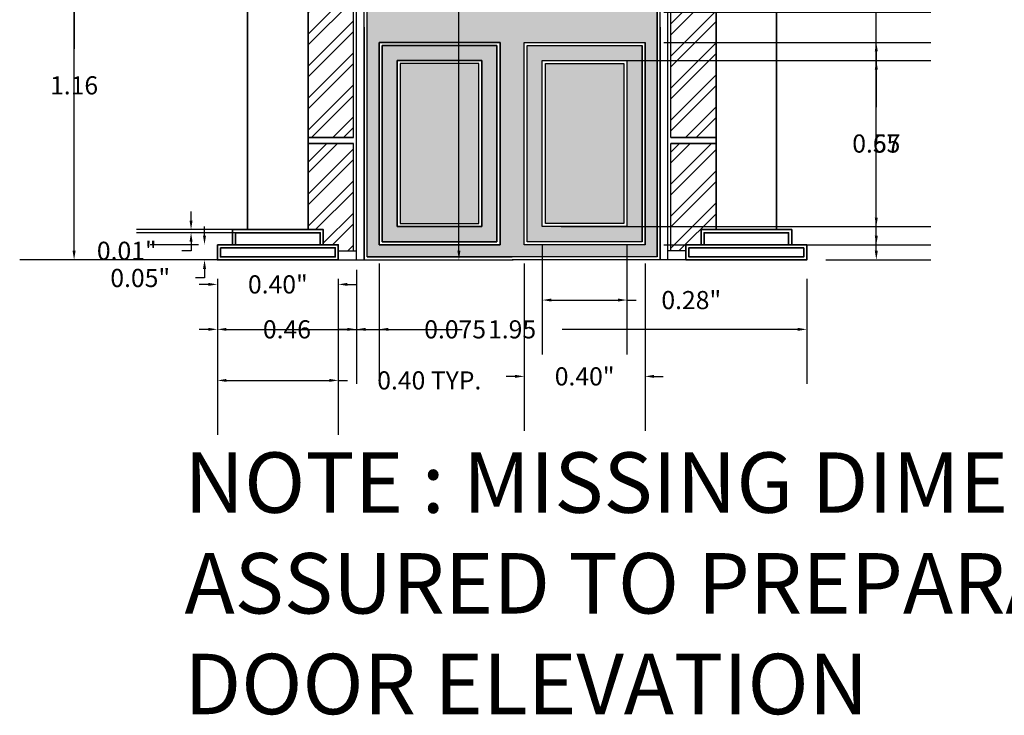
# Model space of a CAD drawing. Units: inches. Extents: x 19.36 to 24.97, y -1.46 to 4.09.
# Tile 1 of 4: x 19.36 to 22.62, y -1.46 to 0.85. Entities that reach past the tile are written whole.
import ezdxf

# ---------------------------------------------------------------- set-up
doc = ezdxf.new("R2010")
doc.units = ezdxf.units.IN
doc.header["$MEASUREMENT"] = 0
for name, color, linetype, lineweight in [('A-ANNO-DIMS', 2, 'Continuous', 18), ('A-ANNO-TEXT', 7, 'Continuous', 25), ('A-COLS', 3, 'Continuous', 35), ('A-DOOR', 4, 'Continuous', 25), ('A-ELEV', 7, 'Continuous', 35), ('A-ELEV-PATT', 8, 'Continuous', 13)]:
    doc.layers.add(name, color=color, linetype=linetype, lineweight=lineweight)
doc.styles.get("Standard").update_dxf_attribs({"font": 'arial.ttf'})
doc.dimstyles.get("Standard").update_dxf_attribs({"dimtxt": 0.06, "dimasz": 0.03, "dimexe": 0.18, "dimexo": 0.0625, "dimgap": 0.09, "dimtad": 0, "dimtih": 1, "dimtoh": 1, "dimzin": 0, "dimdsep": 46, "dimlunit": 3, "dimtxsty": 'Standard', "dimcen": 0, "dimadec": 0, "dimazin": 0, "dimtfac": 1, "dimtofl": 0, "dimtmove": 0, "dimatfit": 3, "dimfxl": 1, "dimtolj": 1, "dimtzin": 0, "dimarcsym": 1})

# ---------------------------------------------------------------- blocks, each defined once
blk = doc.blocks.new('*D10')
at = {"layer": 'A-ANNO-DIMS', "color": 0, "lineweight": -2, "transparency": 16777216}
for p, q in [((21.0886, 0.0975), (21.0886, -0.2631)), ((21.3686, 0.0975), (21.3686, -0.2631)), ((21.1186, -0.0831), (21.3386, -0.0831)), ((21.3686, -0.0831), (21.3986, -0.0831))]:
    blk.add_line(p, q, dxfattribs=at)
at = {"layer": 'A-ANNO-DIMS', "color": 0, "transparency": 16777216}
for points in [[(21.1186, -0.0781), (21.1186, -0.0881), (21.0886, -0.0831)], [(21.3386, -0.0781), (21.3386, -0.0881), (21.3686, -0.0831)]]:
    blk.add_solid(points, dxfattribs=at)
at = {"layer": 'Defpoints', "color": 0, "transparency": 16777216}
for p in [(21.0886, 0.16), (21.3686, 0.16), (21.3686, -0.0831)]:
    blk.add_point(p, dxfattribs=at)
at = {"layer": 'A-ANNO-DIMS', "color": 0, "transparency": 16777216, "insert": (21.5814, -0.0831), "char_height": 0.06, "width": 0.195629, "attachment_point": 5}
blk.add_mtext('\\A1;0.28"', dxfattribs=at)
blk = doc.blocks.new('*D11')
at = {"layer": 'A-ANNO-DIMS', "color": 0, "lineweight": -2, "transparency": 16777216}
for p, q in [((21.0286, 0.0375), (21.0286, -0.5157)), ((21.4286, 0.0375), (21.4286, -0.5157)), ((20.9986, -0.3357), (20.9686, -0.3357)), ((21.4586, -0.3357), (21.4886, -0.3357))]:
    blk.add_line(p, q, dxfattribs=at)
at = {"layer": 'A-ANNO-DIMS', "color": 0, "transparency": 16777216}
for points in [[(20.9986, -0.3307), (20.9986, -0.3407), (21.0286, -0.3357)], [(21.4586, -0.3307), (21.4586, -0.3407), (21.4286, -0.3357)]]:
    blk.add_solid(points, dxfattribs=at)
at = {"layer": 'Defpoints', "color": 0, "transparency": 16777216}
for p in [(21.0286, 0.1), (21.4286, 0.1), (21.4286, -0.3357)]:
    blk.add_point(p, dxfattribs=at)
at = {"layer": 'A-ANNO-DIMS', "color": 0, "transparency": 16777216, "insert": (21.2286, -0.3357), "char_height": 0.06, "attachment_point": 5}
blk.add_mtext('\\A1;0.40"', dxfattribs=at)
blk = doc.blocks.new('*D12')
at = {"layer": 'A-ANNO-DIMS', "color": 0, "lineweight": -2, "transparency": 16777216}
for p, q in [((19.9836, -0.0312), (19.9536, -0.0312)), ((20.0136, -0.0125), (20.0136, -0.2112)), ((20.4136, -0.0125), (20.4136, -0.2112)), ((20.4436, -0.0312), (20.4736, -0.0312))]:
    blk.add_line(p, q, dxfattribs=at)
at = {"layer": 'A-ANNO-DIMS', "color": 0, "transparency": 16777216}
for points in [[(19.9836, -0.0262), (19.9836, -0.0362), (20.0136, -0.0312)], [(20.4436, -0.0262), (20.4436, -0.0362), (20.4136, -0.0312)]]:
    blk.add_solid(points, dxfattribs=at)
at = {"layer": 'Defpoints', "color": 0, "transparency": 16777216}
for p in [(20.0136, 0.05), (20.4136, 0.05), (20.4136, -0.0312)]:
    blk.add_point(p, dxfattribs=at)
at = {"layer": 'A-ANNO-DIMS', "color": 0, "transparency": 16777216, "insert": (20.2136, -0.0312), "char_height": 0.06, "attachment_point": 5}
blk.add_mtext('\\A1;0.40"', dxfattribs=at)
blk = doc.blocks.new('*D13')
at = {"layer": 'A-ANNO-DIMS', "color": 0, "lineweight": -2, "transparency": 16777216}
for p, q in [((19.9709, 0.13), (19.9709, 0.16)), ((19.9511, 0.1), (19.7909, 0.1)), ((19.9511, 0.05), (19.7909, 0.05)), ((19.9709, 0.02), (19.9709, -0.01)), ((19.9709, -0.01), (19.9409, -0.01))]:
    blk.add_line(p, q, dxfattribs=at)
at = {"layer": 'A-ANNO-DIMS', "color": 0, "transparency": 16777216}
for points in [[(19.9659, 0.13), (19.9759, 0.13), (19.9709, 0.1)], [(19.9659, 0.02), (19.9759, 0.02), (19.9709, 0.05)]]:
    blk.add_solid(points, dxfattribs=at)
at = {"layer": 'Defpoints', "color": 0, "transparency": 16777216}
for p in [(20.0136, 0.1), (19.9709, 0.05), (20.0136, 0.05)]:
    blk.add_point(p, dxfattribs=at)
at = {"layer": 'A-ANNO-DIMS', "color": 0, "transparency": 16777216, "insert": (19.7582, -0.01), "char_height": 0.06, "attachment_point": 5}
blk.add_mtext('\\A1;0.05"', dxfattribs=at)
blk = doc.blocks.new('*D14')
at = {"layer": 'A-ANNO-DIMS', "color": 0, "lineweight": -2, "transparency": 16777216}
for p, q in [((19.9264, 0.18), (19.9264, 0.21)), ((20.1322, 0.15), (19.7464, 0.15)), ((20.1322, 0.14), (19.7464, 0.14)), ((19.9264, 0.11), (19.9264, 0.08)), ((19.9264, 0.08), (19.8964, 0.08))]:
    blk.add_line(p, q, dxfattribs=at)
at = {"layer": 'A-ANNO-DIMS', "color": 0, "transparency": 16777216}
for points in [[(19.9214, 0.18), (19.9314, 0.18), (19.9264, 0.15)], [(19.9214, 0.11), (19.9314, 0.11), (19.9264, 0.14)]]:
    blk.add_solid(points, dxfattribs=at)
at = {"layer": 'Defpoints', "color": 0, "transparency": 16777216}
for p in [(19.9264, 0.14), (20.1947, 0.15), (20.1947, 0.14)]:
    blk.add_point(p, dxfattribs=at)
at = {"layer": 'A-ANNO-DIMS', "color": 0, "transparency": 16777216, "insert": (19.7137, 0.08), "char_height": 0.06, "attachment_point": 5}
blk.add_mtext('\\A1;0.01"', dxfattribs=at)
blk = doc.blocks.new('PILASTER')
for p, q in [((20.1136, 2.65), (20.0636, 2.65)), ((20.1136, 2.65), (20.0636, 2.65)), ((20.0636, 2.65), (20.0636, 2.62)), ((20.1136, 2.65), (20.3136, 2.65)), ((20.1136, 2.65), (20.3136, 2.65)), ((20.3136, 2.65), (20.3636, 2.65)), ((20.3136, 2.65), (20.3636, 2.65)), ((20.3636, 2.62), (20.3636, 2.65)), ((20.1136, 2.62), (20.0636, 2.62)), ((20.1136, 2.62), (20.0636, 2.62)), ((20.1136, 2.05), (20.1136, 2.62)), ((20.1136, 2.62), (20.3136, 2.62)), ((20.1136, 2.62), (20.3136, 2.62)), ((20.3136, 2.05), (20.3136, 2.62)), ((20.3136, 2.62), (20.3636, 2.62)), ((20.3136, 2.62), (20.3636, 2.62)), ((20.1136, 1.95), (20.0636, 1.95)), ((20.0636, 1.95), (20.0636, 1.92)), ((20.1136, 1.95), (20.3136, 1.95)), ((20.3136, 1.95), (20.3636, 1.95)), ((20.3636, 1.92), (20.3636, 1.95)), ((20.1136, 1.92), (20.0636, 1.92)), ((20.1136, 0.15), (20.1136, 1.92)), ((20.1136, 1.92), (20.3136, 1.92)), ((20.3136, 0.15), (20.3136, 1.92)), ((20.3136, 1.92), (20.3636, 1.92)), ((20.3136, 0.15), (20.3136, 0.32)), ((20.0636, 0.15), (20.1136, 0.15)), ((20.3636, 0.15), (20.3136, 0.15)), ((20.0136, 0.1), (20.0636, 0.1)), ((20.0136, 0.1), (20.0636, 0.1)), ((20.4136, 0.1), (20.3636, 0.1))]:
    blk.add_line(p, q)
blk.add_lwpolyline([(20.3636, 0.1), (20.3636, 0.15), (20.0636, 0.15), (20.0636, 0.1)])
blk.add_lwpolyline([(20.0136, 0.1), (20.4136, 0.1), (20.4136, 0.05), (20.0136, 0.05)], close=True)
for centre, start, end in [((20.0886, 2.71), 180, 247.3801), ((20.3386, 2.71), 292.6199, 0), ((20.0886, 2.01), 180, 247.3801), ((20.3386, 2.01), 292.6199, 0)]:
    blk.add_arc(centre, 0.065, start, end)
blk = doc.blocks.new('*D17')
at = {"layer": 'A-ANNO-DIMS', "color": 0, "lineweight": -2, "transparency": 16777216}
for p, q in [((20.4761, 2.71), (20.9926, 2.71)), ((20.8126, 2.68), (20.8126, 1.501)), ((20.8126, 0.08), (20.8126, 1.259)), ((20.4761, 0.05), (20.9926, 0.05))]:
    blk.add_line(p, q, dxfattribs=at)
at = {"layer": 'A-ANNO-DIMS', "color": 0, "transparency": 16777216}
for points in [[(20.8076, 2.68), (20.8176, 2.68), (20.8126, 2.71)], [(20.8076, 0.08), (20.8176, 0.08), (20.8126, 0.05)]]:
    blk.add_solid(points, dxfattribs=at)
at = {"layer": 'Defpoints', "color": 0, "transparency": 16777216}
for p in [(20.4136, 2.71), (20.8126, 2.71), (20.4136, 0.05)]:
    blk.add_point(p, dxfattribs=at)
at = {"layer": 'A-ANNO-DIMS', "color": 0, "transparency": 16777216, "insert": (20.8126, 1.38), "char_height": 0.06, "attachment_point": 5}
blk.add_mtext('\\A1;PILASTER 2.66 TYP.', dxfattribs=at)
blk = doc.blocks.new('*D18')
at = {"layer": 'A-ANNO-DIMS', "color": 0, "lineweight": -2, "transparency": 16777216}
for p, q in [((20.0136, -0.0125), (20.0136, -0.529)), ((20.4136, -0.0125), (20.4136, -0.529)), ((20.0436, -0.349), (20.3836, -0.349)), ((20.4136, -0.349), (20.4436, -0.349))]:
    blk.add_line(p, q, dxfattribs=at)
at = {"layer": 'A-ANNO-DIMS', "color": 0, "transparency": 16777216}
for points in [[(20.0436, -0.344), (20.0436, -0.354), (20.0136, -0.349)], [(20.3836, -0.344), (20.3836, -0.354), (20.4136, -0.349)]]:
    blk.add_solid(points, dxfattribs=at)
at = {"layer": 'Defpoints', "color": 0, "transparency": 16777216}
for p in [(20.0136, 0.05), (20.4136, 0.05), (20.4136, -0.349)]:
    blk.add_point(p, dxfattribs=at)
at = {"layer": 'A-ANNO-DIMS', "color": 0, "transparency": 16777216, "insert": (20.7146, -0.349), "char_height": 0.06, "attachment_point": 5}
blk.add_mtext('\\A1;0.40 TYP.', dxfattribs=at)
blk = doc.blocks.new('*D19')
at = {"layer": 'A-ANNO-DIMS', "color": 0, "lineweight": -2, "transparency": 16777216}
for p, q in [((20.0136, -0.0125), (20.0136, -0.36)), ((21.9636, -0.0125), (21.9636, -0.36)), ((20.0436, -0.18), (20.8233, -0.18)), ((21.9336, -0.18), (21.154, -0.18))]:
    blk.add_line(p, q, dxfattribs=at)
at = {"layer": 'A-ANNO-DIMS', "color": 0, "transparency": 16777216}
for points in [[(20.0436, -0.175), (20.0436, -0.185), (20.0136, -0.18)], [(21.9336, -0.175), (21.9336, -0.185), (21.9636, -0.18)]]:
    blk.add_solid(points, dxfattribs=at)
at = {"layer": 'Defpoints', "color": 0, "transparency": 16777216}
for p in [(20.0136, 0.05), (21.9636, 0.05), (21.9636, -0.18)]:
    blk.add_point(p, dxfattribs=at)
at = {"layer": 'A-ANNO-DIMS', "color": 0, "transparency": 16777216, "insert": (20.9886, -0.18), "char_height": 0.06, "attachment_point": 5}
blk.add_mtext('\\A1;1.95', dxfattribs=at)
blk = doc.blocks.new('*D20')
at = {"layer": 'A-ANNO-DIMS', "color": 0, "lineweight": -2, "transparency": 16777216}
for p, q in [((21.0509, 3.5451), (22.3736, 3.5451)), ((22.1936, 3.5151), (22.1936, 1.9182)), ((22.1936, 0.08), (22.1936, 1.6769)), ((22.0261, 0.05), (22.3736, 0.05))]:
    blk.add_line(p, q, dxfattribs=at)
at = {"layer": 'A-ANNO-DIMS', "color": 0, "transparency": 16777216}
for points in [[(22.1886, 3.5151), (22.1986, 3.5151), (22.1936, 3.5451)], [(22.1886, 0.08), (22.1986, 0.08), (22.1936, 0.05)]]:
    blk.add_solid(points, dxfattribs=at)
at = {"layer": 'Defpoints', "color": 0, "transparency": 16777216}
for p in [(20.9884, 3.5451), (22.1936, 3.5451), (21.9636, 0.05)]:
    blk.add_point(p, dxfattribs=at)
at = {"layer": 'A-ANNO-DIMS', "color": 0, "transparency": 16777216, "insert": (22.1936, 1.7976), "char_height": 0.06, "attachment_point": 5}
blk.add_mtext('\\A1;3.495', dxfattribs=at)
blk = doc.blocks.new('*D21')
at = {"layer": 'A-ANNO-DIMS', "color": 0, "lineweight": -2, "transparency": 16777216}
for p, q in [((20.4736, 0.1125), (20.4736, 4.0914)), ((21.5036, 0.1125), (21.5036, 4.0914)), ((20.5036, 3.9114), (20.8235, 3.9114)), ((21.4736, 3.9114), (21.1537, 3.9114))]:
    blk.add_line(p, q, dxfattribs=at)
at = {"layer": 'A-ANNO-DIMS', "color": 0, "transparency": 16777216}
for points in [[(20.5036, 3.9164), (20.5036, 3.9064), (20.4736, 3.9114)], [(21.4736, 3.9164), (21.4736, 3.9064), (21.5036, 3.9114)]]:
    blk.add_solid(points, dxfattribs=at)
at = {"layer": 'Defpoints', "color": 0, "transparency": 16777216}
for p in [(21.5036, 3.9114), (20.4736, 0.05), (21.5036, 0.05)]:
    blk.add_point(p, dxfattribs=at)
at = {"layer": 'A-ANNO-DIMS', "color": 0, "transparency": 16777216, "insert": (20.9886, 3.9114), "char_height": 0.06, "attachment_point": 5}
blk.add_mtext('\\A1;1.03', dxfattribs=at)
blk = doc.blocks.new('*D22')
at = {"layer": 'A-ANNO-DIMS', "color": 0, "lineweight": -2, "transparency": 16777216}
for p, q in [((20.013629, -0.012487), (20.013629, -0.359987)), ((20.473629, -0.012487), (20.473629, -0.359987)), ((19.983629, -0.179987), (19.953629, -0.179987)), ((20.503629, -0.179987), (20.533629, -0.179987))]:
    blk.add_line(p, q, dxfattribs=at)
at = {"layer": 'A-ANNO-DIMS', "color": 0, "transparency": 16777216}
for points in [[(19.983629, -0.174987), (19.983629, -0.184987), (20.013629, -0.179987)], [(20.503629, -0.174987), (20.503629, -0.184987), (20.473629, -0.179987)]]:
    blk.add_solid(points, dxfattribs=at)
at = {"layer": 'Defpoints', "color": 0, "transparency": 16777216}
for p in [(20.013629, 0.050013), (20.473629, 0.050013), (20.473629, -0.179987)]:
    blk.add_point(p, dxfattribs=at)
at = {"layer": 'A-ANNO-DIMS', "color": 0, "transparency": 16777216, "insert": (20.243629, -0.179987), "char_height": 0.06, "attachment_point": 5}
blk.add_mtext('\\A1;0.46', dxfattribs=at)
blk = doc.blocks.new('*D23')
at = {"layer": 'A-ANNO-DIMS', "color": 0, "lineweight": -2, "transparency": 16777216}
for p, q in [((20.9261, 1.2054), (19.3594, 1.2054)), ((19.5394, 1.1754), (19.5394, 0.7483)), ((19.5394, 0.08), (19.5394, 0.5071)), ((20.4111, 0.05), (19.3594, 0.05))]:
    blk.add_line(p, q, dxfattribs=at)
at = {"layer": 'A-ANNO-DIMS', "color": 0, "transparency": 16777216}
for points in [[(19.5344, 1.1754), (19.5444, 1.1754), (19.5394, 1.2054)], [(19.5344, 0.08), (19.5444, 0.08), (19.5394, 0.05)]]:
    blk.add_solid(points, dxfattribs=at)
at = {"layer": 'Defpoints', "color": 0, "transparency": 16777216}
for p in [(19.5394, 1.2054), (20.9886, 1.2054), (20.4736, 0.05)]:
    blk.add_point(p, dxfattribs=at)
at = {"layer": 'A-ANNO-DIMS', "color": 0, "transparency": 16777216, "insert": (19.5394, 0.6277), "char_height": 0.06, "attachment_point": 5}
blk.add_mtext('\\A1;1.16', dxfattribs=at)
blk = doc.blocks.new('*D26')
at = {"layer": 'A-ANNO-DIMS', "color": 0, "lineweight": -2, "transparency": 16777216}
for p, q in [((19.9511, 2.75), (19.3594, 2.75)), ((19.5394, 2.72), (19.5394, 1.5206)), ((19.5394, 0.08), (19.5394, 1.2794)), ((19.9511, 0.05), (19.3594, 0.05))]:
    blk.add_line(p, q, dxfattribs=at)
at = {"layer": 'A-ANNO-DIMS', "color": 0, "transparency": 16777216}
for points in [[(19.5344, 2.72), (19.5444, 2.72), (19.5394, 2.75)], [(19.5344, 0.08), (19.5444, 0.08), (19.5394, 0.05)]]:
    blk.add_solid(points, dxfattribs=at)
at = {"layer": 'Defpoints', "color": 0, "transparency": 16777216}
for p in [(19.5394, 2.75), (20.0136, 2.75), (20.0136, 0.05)]:
    blk.add_point(p, dxfattribs=at)
at = {"layer": 'A-ANNO-DIMS', "color": 0, "transparency": 16777216, "insert": (19.5394, 1.4), "char_height": 0.06, "attachment_point": 5}
blk.add_mtext('\\A1;2.70', dxfattribs=at)
blk = doc.blocks.new('*D27')
at = {"layer": 'A-ANNO-DIMS', "color": 0, "lineweight": -2, "transparency": 16777216}
for p, q in [((19.9523, 2.9877), (19.3594, 2.9877)), ((19.5394, 2.9577), (19.5394, 1.6395)), ((19.5394, 0.08), (19.5394, 1.3982)), ((19.9511, 0.05), (19.3594, 0.05))]:
    blk.add_line(p, q, dxfattribs=at)
at = {"layer": 'A-ANNO-DIMS', "color": 0, "transparency": 16777216}
for points in [[(19.5344, 2.9577), (19.5444, 2.9577), (19.5394, 2.9877)], [(19.5344, 0.08), (19.5444, 0.08), (19.5394, 0.05)]]:
    blk.add_solid(points, dxfattribs=at)
at = {"layer": 'Defpoints', "color": 0, "transparency": 16777216}
for p in [(20.0148, 2.9877), (19.5394, 0.05), (20.0136, 0.05)]:
    blk.add_point(p, dxfattribs=at)
at = {"layer": 'A-ANNO-DIMS', "color": 0, "transparency": 16777216, "insert": (19.5394, 1.5189), "char_height": 0.06, "attachment_point": 5}
blk.add_mtext('\\A1;2.938', dxfattribs=at)
blk = doc.blocks.new('*D29')
at = {"layer": 'A-ANNO-DIMS', "color": 0, "lineweight": -2, "transparency": 16777216}
for p, q in [((21.4911, 0.77), (22.3736, 0.77)), ((22.1936, 0.74), (22.1936, 0.5556)), ((22.1936, 0.13), (22.1936, 0.3144)), ((21.4911, 0.1), (22.3736, 0.1))]:
    blk.add_line(p, q, dxfattribs=at)
at = {"layer": 'A-ANNO-DIMS', "color": 0, "transparency": 16777216}
for points in [[(22.1886, 0.74), (22.1986, 0.74), (22.1936, 0.77)], [(22.1886, 0.13), (22.1986, 0.13), (22.1936, 0.1)]]:
    blk.add_solid(points, dxfattribs=at)
at = {"layer": 'Defpoints', "color": 0, "transparency": 16777216}
for p in [(21.4286, 0.77), (22.1936, 0.77), (21.4286, 0.1)]:
    blk.add_point(p, dxfattribs=at)
at = {"layer": 'A-ANNO-DIMS', "color": 0, "transparency": 16777216, "insert": (22.1936, 0.435), "char_height": 0.06, "attachment_point": 5}
blk.add_mtext('\\A1;0.67', dxfattribs=at)
blk = doc.blocks.new('*D30')
at = {"layer": 'A-ANNO-DIMS', "color": 0, "lineweight": -2, "transparency": 16777216}
for p, q in [((22.1936, 0.9), (22.1936, 0.93)), ((22.1936, 0.93), (22.2236, 0.93)), ((21.4911, 0.87), (22.3736, 0.87)), ((21.4911, 0.77), (22.3736, 0.77)), ((22.1936, 0.74), (22.1936, 0.71))]:
    blk.add_line(p, q, dxfattribs=at)
at = {"layer": 'A-ANNO-DIMS', "color": 0, "transparency": 16777216}
for points in [[(22.1886, 0.9), (22.1986, 0.9), (22.1936, 0.87)], [(22.1886, 0.74), (22.1986, 0.74), (22.1936, 0.77)]]:
    blk.add_solid(points, dxfattribs=at)
at = {"layer": 'Defpoints', "color": 0, "transparency": 16777216}
for p in [(21.4286, 0.87), (22.1936, 0.87), (21.4286, 0.77)]:
    blk.add_point(p, dxfattribs=at)
at = {"layer": 'A-ANNO-DIMS', "color": 0, "transparency": 16777216, "insert": (22.3915, 0.93), "char_height": 0.06, "attachment_point": 5}
blk.add_mtext('\\A1;0.10', dxfattribs=at)
blk = doc.blocks.new('*D32')
at = {"layer": 'A-ANNO-DIMS', "color": 0, "lineweight": -2, "transparency": 16777216}
for p, q in [((21.1511, 0.71), (22.3736, 0.71)), ((22.1936, 0.68), (22.1936, 0.5556)), ((22.1936, 0.19), (22.1936, 0.3144)), ((21.1511, 0.16), (22.3736, 0.16))]:
    blk.add_line(p, q, dxfattribs=at)
at = {"layer": 'A-ANNO-DIMS', "color": 0, "transparency": 16777216}
for points in [[(22.1886, 0.68), (22.1986, 0.68), (22.1936, 0.71)], [(22.1886, 0.19), (22.1986, 0.19), (22.1936, 0.16)]]:
    blk.add_solid(points, dxfattribs=at)
at = {"layer": 'Defpoints', "color": 0, "transparency": 16777216}
for p in [(21.0886, 0.71), (22.1936, 0.71), (21.0886, 0.16)]:
    blk.add_point(p, dxfattribs=at)
at = {"layer": 'A-ANNO-DIMS', "color": 0, "transparency": 16777216, "insert": (22.1936, 0.435), "char_height": 0.06, "attachment_point": 5}
blk.add_mtext('\\A1;0.55', dxfattribs=at)
blk = doc.blocks.new('*D34')
at = {"layer": 'A-ANNO-DIMS', "color": 0, "lineweight": -2, "transparency": 16777216}
for p, q in [((20.5486, 0.0375), (20.5486, -0.36)), ((20.4736, 0.0175), (20.4736, -0.36)), ((20.4436, -0.18), (20.4136, -0.18)), ((20.5786, -0.18), (20.6086, -0.18))]:
    blk.add_line(p, q, dxfattribs=at)
at = {"layer": 'A-ANNO-DIMS', "color": 0, "transparency": 16777216}
for points in [[(20.4436, -0.175), (20.4436, -0.185), (20.4736, -0.18)], [(20.5786, -0.175), (20.5786, -0.185), (20.5486, -0.18)]]:
    blk.add_solid(points, dxfattribs=at)
at = {"layer": 'Defpoints', "color": 0, "transparency": 16777216}
for p in [(20.5486, 0.1), (20.4736, 0.08), (20.5486, -0.18)]:
    blk.add_point(p, dxfattribs=at)
at = {"layer": 'A-ANNO-DIMS', "color": 0, "transparency": 16777216, "insert": (20.8001, -0.18), "char_height": 0.06, "attachment_point": 5}
blk.add_mtext('\\A1;0.075', dxfattribs=at)

msp = doc.modelspace()

# ---------------------------------------------------------------- hatches: boundary and pattern name
at = {"layer": 'A-ELEV-PATT'}
h = msp.add_hatch(dxfattribs=at)
h.set_pattern_fill('ANSI32', color=256, scale=0.2)
h.paths.add_polyline_path([(20.6294, 2.4913, 0.064491), (20.3136, 2.3574), (20.3136, 2.2989), (20.4636, 2.2231, -0.061889), (20.7287, 2.3207)])
h.paths.add_polyline_path([(20.9886, 2.5406, 0.066262), (20.6394, 2.4941), (20.7389, 2.323, -0.055018), (20.9886, 2.3506)])
h.paths.add_polyline_path([(21.3488, 2.491, 0.066519), (20.9986, 2.5405), (20.9986, 2.3505, -0.055118), (21.2486, 2.3207)])
h.paths.add_polyline_path([(21.6636, 2.3574, 0.062356), (21.3588, 2.4882), (21.2588, 2.3182, -0.0596), (21.5136, 2.2231), (21.6636, 2.2812)])
h.paths.add_polyline_path([(21.6636, 2.2704), (21.5136, 2.2124), (21.5136, 2.1846), (21.5136, 1.5166), (21.6636, 1.5166), (21.6636, 1.92), (21.6136, 1.92), (21.6136, 1.95, -0.261087), (21.5744, 2), (21.5636, 2), (21.5636, 2.05), (21.6136, 2.05), (21.6636, 2.05)])
h.paths.add_polyline_path([(21.6636, 1.4966), (21.5136, 1.4966), (21.5136, 0.9758), (21.6636, 0.9758)])
h.paths.add_polyline_path([(21.6636, 0.9558), (21.5136, 0.9558), (21.5136, 0.455), (21.6636, 0.455)])
h.paths.add_polyline_path([(21.6636, 0.435), (21.5136, 0.435), (21.5136, 0.08), (21.5636, 0.08), (21.5636, 0.1), (21.6136, 0.1), (21.6136, 0.15), (21.6636, 0.15)])
h.paths.add_polyline_path([(20.4636, 0.435), (20.3136, 0.435), (20.3136, 0.15), (20.3636, 0.15), (20.3636, 0.1), (20.4136, 0.1), (20.4136, 0.08), (20.4636, 0.08)])
h.paths.add_polyline_path([(20.4636, 0.9558), (20.3136, 0.9558), (20.3136, 0.455), (20.4636, 0.455)])
h.paths.add_polyline_path([(20.4636, 1.4966), (20.3136, 1.4966), (20.3136, 0.9758), (20.4636, 0.9758)])
h.paths.add_polyline_path([(20.4636, 2.1846), (20.4636, 2.2119), (20.3136, 2.2877), (20.3136, 2.05), (20.3636, 2.05), (20.4136, 2.05), (20.4136, 2), (20.4029, 2, -0.261087), (20.3636, 1.95), (20.3636, 1.92), (20.3136, 1.92), (20.3136, 1.5166), (20.4636, 1.5166)])
h = msp.add_hatch(color=256, dxfattribs=at)
h.dxf.hatch_style = 1
h.paths.add_polyline_path([(21.3586, 2.0968, 0.070017), (21.0982, 2.1643), (21.0986, 0.94), (21.3586, 0.94)], flags=0)
h.paths.add_polyline_path([(20.8785, 2.1642, 0.070014), (20.6181, 2.0966), (20.6186, 0.94), (20.8786, 0.94)], flags=0)
h.paths.add_polyline_path([(21.4686, 2.1786, 0.115049), (20.9886, 2.2906, 0.115049), (20.5086, 2.1786), (20.5086, 0.06), (20.8541, 0.06), (20.9886, 0.06), (21.1231, 0.06), (21.4686, 0.06)])
h.paths.add_polyline_path([(21.0282, 2.2398, -0.100527), (21.4286, 2.1424), (21.4286, 0.87), (21.0286, 0.87)], flags=16)
h.paths.add_polyline_path([(21.0382, 2.2294, -0.096406), (21.4186, 2.136), (21.4186, 0.88), (21.0386, 0.88)], flags=0)
h.paths.add_polyline_path([(20.9486, 0.87), (20.5484, 0.87), (20.5476, 2.1419, -0.10066), (20.9485, 2.2398)], flags=16)
h.paths.add_polyline_path([(20.9386, 0.88), (20.5586, 0.88), (20.5581, 2.1358, -0.096404), (20.9385, 2.2293)], flags=0)
h.paths.add_polyline_path([(21.0882, 2.1755, -0.074627), (21.3686, 2.1035), (21.3686, 0.93), (21.0886, 0.93)], flags=0)
h.paths.add_polyline_path([(21.0982, 2.1643, -0.070017), (21.3586, 2.0968), (21.3586, 0.94), (21.0986, 0.94)], flags=0)
h.paths.add_polyline_path([(20.8886, 0.93), (20.6086, 0.93), (20.6081, 2.1032, -0.074624), (20.8885, 2.1754)], flags=0)
h.paths.add_polyline_path([(20.8786, 0.94), (20.6186, 0.94), (20.6181, 2.0966, -0.070014), (20.8785, 2.1642)], flags=0)
h.paths.add_polyline_path([(21.0286, 0.77), (21.4286, 0.77), (21.4286, 0.1), (21.0286, 0.1)], flags=16)
h.paths.add_polyline_path([(20.9486, 0.77), (20.9486, 0.1), (20.5486, 0.1), (20.5486, 0.77)], flags=16)
h.paths.add_polyline_path([(21.0386, 0.76), (21.4186, 0.76), (21.4186, 0.11), (21.0386, 0.11)], flags=0)
h.paths.add_polyline_path([(20.9386, 0.76), (20.9386, 0.11), (20.5586, 0.11), (20.5586, 0.76)], flags=0)
h.paths.add_polyline_path([(21.0886, 0.71), (21.3686, 0.71), (21.3686, 0.16), (21.0886, 0.16)], flags=0)
h.paths.add_polyline_path([(20.8886, 0.71), (20.8886, 0.16), (20.6086, 0.16), (20.6086, 0.71)], flags=0)
h.paths.add_polyline_path([(21.0986, 0.7), (21.3586, 0.7), (21.3586, 0.17), (21.0986, 0.17)], flags=0)
h.paths.add_polyline_path([(20.8786, 0.7), (20.8786, 0.17), (20.6186, 0.17), (20.6186, 0.7)], flags=0)
h.paths.add_polyline_path([(21.3586, 0.7), (21.0986, 0.7), (21.0986, 0.17), (21.3586, 0.17)], flags=0)
h = msp.add_hatch(color=256, dxfattribs=at)
h.dxf.hatch_style = 1
h.paths.add_polyline_path([(20.8785, 2.1642, 0.070014), (20.6181, 2.0966), (20.6186, 0.94), (20.8786, 0.94)], flags=0)
h.paths.add_polyline_path([(20.9385, 2.2293, 0.096404), (20.5581, 2.1358), (20.5586, 0.88), (20.9386, 0.88)])
h.paths.add_polyline_path([(20.6086, 0.93), (20.8886, 0.93), (20.8885, 2.1754, 0.074624), (20.6081, 2.1032)], flags=16)
h.paths.add_polyline_path([(20.6181, 2.0966, -0.070014), (20.8785, 2.1642), (20.8786, 0.94), (20.6186, 0.94)], flags=0)
h.paths.add_polyline_path([(21.4186, 2.136, 0.096406), (21.0382, 2.2294), (21.0386, 0.88), (21.4186, 0.88)])
h.paths.add_polyline_path([(21.0882, 2.1755, -0.074627), (21.3686, 2.1035), (21.3686, 0.93), (21.0886, 0.93)], flags=16)
h.paths.add_polyline_path([(21.0982, 2.1643, -0.070017), (21.3586, 2.0968), (21.3586, 0.94), (21.0986, 0.94)], flags=0)
h.paths.add_polyline_path([(21.4186, 0.76), (21.0386, 0.76), (21.0386, 0.11), (21.4186, 0.11)])
h.paths.add_polyline_path([(21.0886, 0.71), (21.3686, 0.71), (21.3686, 0.16), (21.0886, 0.16)], flags=16)
h.paths.add_polyline_path([(21.0986, 0.7), (21.3586, 0.7), (21.3586, 0.17), (21.0986, 0.17)], flags=0)
h.paths.add_polyline_path([(20.9386, 0.76), (20.5586, 0.76), (20.5586, 0.11), (20.9386, 0.11)])
h.paths.add_polyline_path([(20.8886, 0.16), (20.6086, 0.16), (20.6086, 0.71), (20.8886, 0.71)], flags=16)
h.paths.add_polyline_path([(20.8786, 0.17), (20.6186, 0.17), (20.6186, 0.7), (20.8786, 0.7)], flags=0)
h = msp.add_hatch(color=256, dxfattribs=at)
h.dxf.hatch_style = 1
h.paths.add_polyline_path([(21.3586, 2.0968, 0.070017), (21.0982, 2.1643), (21.0986, 0.94), (21.3586, 0.94)])
h.paths.add_polyline_path([(21.3586, 0.7), (21.0986, 0.7), (21.0986, 0.17), (21.3586, 0.17)])
h.paths.add_polyline_path([(20.8785, 2.1642, 0.070014), (20.6181, 2.0966), (20.6186, 0.94), (20.8786, 0.94)])
h.paths.add_polyline_path([(20.8786, 0.7), (20.6186, 0.7), (20.6186, 0.17), (20.8786, 0.17)])

# ---------------------------------------------------------------- linework, layer by layer
at = {"layer": 'A-DOOR'}
for p, q in [((20.4986, 0.82), (20.4986, 0.05)), ((21.4786, 0.82), (21.4786, 0.05)), ((20.5486, 0.77), (20.5486, 0.1)), ((20.9486, 0.77), (20.5486, 0.77)), ((20.9486, 0.1), (20.9486, 0.77)), ((21.0286, 0.1), (21.0286, 0.77)), ((21.0286, 0.77), (21.4286, 0.77)), ((21.4286, 0.77), (21.4286, 0.1)), ((20.5486, 0.1), (20.9486, 0.1)), ((21.4286, 0.1), (21.0286, 0.1)), ((20.4136, 0.08), (20.4636, 0.08)), ((20.4636, 0.08), (20.4736, 0.08)), ((21.5136, 0.08), (21.5036, 0.08)), ((21.5636, 0.08), (21.5136, 0.08)), ((20.4136, 0.05), (20.4636, 0.05)), ((20.4636, 0.05), (20.4736, 0.05)), ((20.4736, 0.05), (20.9886, 0.05)), ((20.4986, 0.05), (20.9736, 0.05)), ((21.5036, 0.05), (20.9886, 0.05)), ((21.4786, 0.05), (21.0036, 0.05)), ((21.5136, 0.05), (21.5036, 0.05)), ((21.5636, 0.05), (21.5136, 0.05))]:
    msp.add_line(p, q, dxfattribs=at)
for points in [[(20.4736, 0.05), (20.4736, 2.1913)], [(20.4986, 0.05), (20.4986, 2.1848)], [(21.4786, 0.05), (21.4786, 2.1848)], [(21.5036, 0.05), (21.5036, 2.1913)], [(20.5086, 0.06), (20.5086, 2.1786)], [(21.4686, 2.1786), (21.4686, 0.06), (20.5086, 0.06)], [(21.4686, 0.06), (21.4686, 2.1786)], [(20.4636, 0.455), (20.4636, 0.9558)], [(21.5136, 0.455), (21.5136, 0.9558)], [(20.5486, 0.77), (20.9486, 0.77), (20.9486, 0.1), (20.5486, 0.1), (20.5486, 0.77)], [(20.5586, 0.76), (20.9386, 0.76), (20.9386, 0.11), (20.5586, 0.11), (20.5586, 0.76)], [(21.4186, 0.11), (21.4186, 0.76)], [(21.4286, 0.1), (21.4286, 0.77)], [(20.6086, 0.71), (20.8886, 0.71), (20.8886, 0.16), (20.6086, 0.16), (20.6086, 0.71)], [(20.4636, 0.08), (20.4636, 0.435)], [(21.5136, 0.08), (21.5136, 0.435)], [(20.4736, 0.05), (20.8541, 0.05)], [(20.5086, 0.06), (20.8541, 0.06)], [(20.8541, 0.06), (20.9886, 0.06)], [(20.8541, 0.05), (20.9736, 0.05)], [(21.1231, 0.06), (20.9886, 0.06)], [(21.1231, 0.05), (21.0036, 0.05)], [(21.4686, 0.06), (21.1231, 0.06)], [(21.5036, 0.05), (21.1231, 0.05)]]:
    msp.add_lwpolyline(points, dxfattribs=at)
for points in [[(20.5586, 0.76), (20.5586, 0.11), (20.9386, 0.11), (20.9386, 0.76)], [(21.4186, 0.76), (21.4186, 0.11), (21.0386, 0.11), (21.0386, 0.76)], [(20.6086, 0.71), (20.6086, 0.16), (20.8886, 0.16), (20.8886, 0.71)], [(20.6186, 0.7), (20.6186, 0.17), (20.8786, 0.17), (20.8786, 0.7)], [(21.3686, 0.71), (21.3686, 0.16), (21.0886, 0.16), (21.0886, 0.71)], [(21.3586, 0.7), (21.3586, 0.17), (21.0986, 0.17), (21.0986, 0.7)]]:
    msp.add_lwpolyline(points, close=True, dxfattribs=at)
at = {"layer": 'A-ELEV'}
for p, q in [((20.4636, 0.455), (20.3136, 0.455)), ((20.3136, 0.455), (20.4636, 0.455)), ((20.4636, 0.435), (20.3136, 0.435)), ((20.3136, 0.435), (20.4636, 0.435)), ((21.5136, 0.455), (21.6636, 0.455)), ((21.5136, 0.435), (21.6636, 0.435))]:
    msp.add_line(p, q, dxfattribs=at)
for points in [[(20.3536, 0.1), (20.3536, 0.14), (20.0736, 0.14), (20.0736, 0.1)], [(21.6236, 0.1), (21.6236, 0.14), (21.9036, 0.14), (21.9036, 0.1)], [(20.3136, 0.1), (20.1136, 0.1)], [(21.6636, 0.1), (21.8636, 0.1)]]:
    msp.add_lwpolyline(points, dxfattribs=at)
for points in [[(20.0236, 0.09), (20.4036, 0.09), (20.4036, 0.06), (20.0236, 0.06)], [(21.9536, 0.09), (21.5736, 0.09), (21.5736, 0.06), (21.9536, 0.06)]]:
    msp.add_lwpolyline(points, close=True, dxfattribs=at)

# ---------------------------------------------------------------- block references
at = {"layer": 'A-COLS'}
msp.add_blockref('PILASTER', (0, 0), dxfattribs=at)
at = {"layer": 'A-COLS', "extrusion": (0, 0, -1), "zscale": -1}
msp.add_blockref('PILASTER', (-41.9773, 0), dxfattribs=at)

# ---------------------------------------------------------------- texts
at = {"layer": 'A-ANNO-TEXT', "insert": (19.9047, -0.5872), "char_height": 0.2, "attachment_point": 1}
msp.add_mtext_dynamic_manual_height_columns('NOTE : MISSING DIMENSIONS TO BE ASSURED TO PREPARATION BY DRAWER DOOR ELEVATION', width=5.813598, gutter_width=1, heights=[0], dxfattribs=at)

# ---------------------------------------------------------------- dimensions: what is measured, and where the dimension line sits
at = {"layer": 'A-ANNO-DIMS'}
for base, p1, p2, override, picture, middle in [((21.5036, 3.9114), (20.4736, 0.05), (21.5036, 0.05), {"dimdec": 2, "dimlfac": 1, "dimrnd": 0, "dimzin": 0, "dimdsep": 46, "dimlunit": 2}, '*D21', (20.9886, 3.9114)), ((21.3686, -0.0831), (21.0886, 0.16), (21.3686, 0.16), {"dimclrd": 0, "dimclre": 0, "dimclrt": 0}, '*D10', (21.5814, -0.0831)), ((20.5486, -0.18), (20.4736, 0.08), (20.5486, 0.1), {"dimdec": 3, "dimlfac": 1, "dimrnd": 0, "dimzin": 0, "dimdsep": 46, "dimlunit": 2}, '*D34', (20.8001, -0.18)), ((21.4286, -0.3357), (21.0286, 0.1), (21.4286, 0.1), {"dimclrd": 0, "dimclre": 0, "dimclrt": 0}, '*D11', (21.2286, -0.3357)), ((20.4136, -0.0312), (20.0136, 0.05), (20.4136, 0.05), {"dimclrd": 0, "dimclre": 0, "dimclrt": 0}, '*D12', (20.2136, -0.0312)), ((20.4736, -0.18), (20.0136, 0.05), (20.4736, 0.05), {"dimdec": 2, "dimlfac": 1, "dimrnd": 0, "dimzin": 0, "dimdsep": 46, "dimlunit": 2}, '*D22', (20.2436, -0.18)), ((21.9636, -0.18), (20.0136, 0.05), (21.9636, 0.05), {"dimdec": 2, "dimlfac": 1, "dimrnd": 0, "dimzin": 0, "dimdsep": 46, "dimlunit": 2}, '*D19', (20.9886, -0.18))]:
    dim = msp.add_linear_dim(base=base, p1=p1, p2=p2, dimstyle='Standard', override=override, dxfattribs=at)
    dim.commit()
    dim.dimension.update_dxf_attribs({"geometry": picture, "text_midpoint": middle})
for base, p1, p2, override, picture, middle in [((22.1936, 3.5451), (21.9636, 0.05), (20.9884, 3.5451), {"dimdec": 3, "dimlfac": 1, "dimrnd": 0, "dimzin": 0, "dimdsep": 46, "dimlunit": 2}, '*D20', (22.1936, 1.7976)), ((19.5394, 0.05), (20.0148, 2.9877), (20.0136, 0.05), {"dimdec": 3, "dimlfac": 1, "dimrnd": 0, "dimzin": 0, "dimdsep": 46, "dimlunit": 2}, '*D27', (19.5394, 1.5189)), ((19.5394, 2.75), (20.0136, 0.05), (20.0136, 2.75), {"dimdec": 2, "dimlfac": 1, "dimrnd": 0, "dimzin": 0, "dimdsep": 46, "dimlunit": 2}, '*D26', (19.5394, 1.4)), ((19.5394, 1.2054), (20.4736, 0.05), (20.9886, 1.2054), {"dimdec": 2, "dimlfac": 1, "dimrnd": 0, "dimzin": 0, "dimdsep": 46, "dimlunit": 2}, '*D23', (19.5394, 0.6277)), ((22.1936, 0.87), (21.4286, 0.77), (21.4286, 0.87), {"dimdec": 2, "dimlfac": 1, "dimrnd": 0, "dimzin": 0, "dimdsep": 46, "dimlunit": 2}, '*D30', (22.3915, 0.93)), ((22.1936, 0.77), (21.4286, 0.1), (21.4286, 0.77), {"dimdec": 2, "dimlfac": 1, "dimrnd": 0, "dimzin": 0, "dimdsep": 46, "dimlunit": 2}, '*D29', (22.1936, 0.435)), ((22.1936, 0.71), (21.0886, 0.16), (21.0886, 0.71), {"dimdec": 2, "dimlfac": 1, "dimrnd": 0, "dimzin": 0, "dimdsep": 46, "dimlunit": 2}, '*D32', (22.1936, 0.435)), ((19.9264, 0.14), (20.1947, 0.15), (20.1947, 0.14), {"dimclrd": 0, "dimclre": 0, "dimclrt": 0}, '*D14', (19.7137, 0.08)), ((19.9709, 0.05), (20.0136, 0.1), (20.0136, 0.05), {"dimclrd": 0, "dimclre": 0, "dimclrt": 0}, '*D13', (19.7582, -0.01))]:
    dim = msp.add_linear_dim(base=base, p1=p1, p2=p2, angle=90, dimstyle='Standard', override=override, dxfattribs=at)
    dim.commit()
    dim.dimension.update_dxf_attribs({"geometry": picture, "text_midpoint": middle})
dim = msp.add_linear_dim(base=(20.8126, 2.71), p1=(20.4136, 0.05), p2=(20.4136, 2.71), angle=90, text='PILASTER <> TYP.', dimstyle='Standard', override={"dimdec": 2, "dimrnd": 0, "dimzin": 0, "dimlunit": 2}, dxfattribs=at)
dim.commit()
dim.dimension.update_dxf_attribs({"geometry": '*D17', "text_midpoint": (20.8126, 1.38)})
dim = msp.add_linear_dim(base=(20.4136, -0.349), p1=(20.0136, 0.05), p2=(20.4136, 0.05), text='<> TYP.', dimstyle='Standard', override={"dimdec": 2, "dimrnd": 0, "dimzin": 0, "dimlunit": 2}, dxfattribs=at)
dim.commit()
dim.dimension.update_dxf_attribs({"geometry": '*D18', "text_midpoint": (20.7146, -0.349)})

doc.saveas('drawing.dxf')
